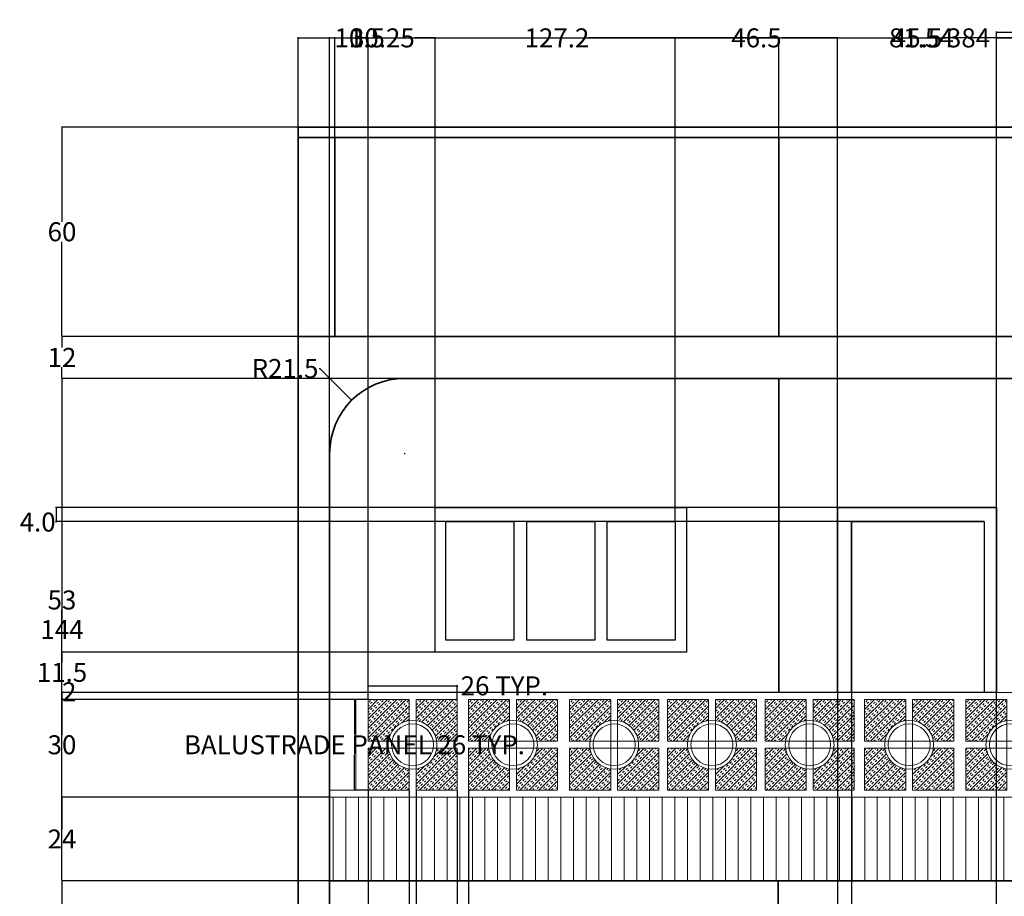
# Model space of a CAD drawing. Units: inches. Extents: x 12 to 590, y 127 to 569.
# Tile 2 of 4: x 12 to 294, y 318 to 569. Entities that reach past the tile are written whole.
import ezdxf

# ---------------------------------------------------------------- set-up
doc = ezdxf.new("R2010")
doc.units = ezdxf.units.IN
doc.header["$MEASUREMENT"] = 0
for name, color, linetype, lineweight in [('A-ANNO-DIMS', 2, 'Continuous', 18), ('A-DETL-RAIL', 6, 'Continuous', 18), ('A-DOOR', 3, 'Continuous', 25), ('A-ELEV', 7, 'Continuous', 35), ('A-GLAZ', 4, 'Continuous', 25), ('A-WALL-PATT', 8, 'Continuous', 13)]:
    doc.layers.add(name, color=color, linetype=linetype, lineweight=lineweight)
doc.styles.get("Standard").update_dxf_attribs({"font": 'arial.ttf'})
doc.dimstyles.get("Standard").update_dxf_attribs({"dimtxt": 5.4375, "dimasz": 0.18, "dimexe": 0.18, "dimexo": 0.0625, "dimgap": 0.09, "dimtad": 0, "dimtih": 1, "dimtoh": 1, "dimdec": 4, "dimzin": 0, "dimdsep": 46, "dimlunit": 4, "dimtxsty": 'Standard', "dimcen": 0.09, "dimadec": 0, "dimazin": 0, "dimtfac": 1, "dimtdec": 4, "dimtofl": 0, "dimtmove": 0, "dimatfit": 3, "dimfxl": 1, "dimtolj": 1, "dimtzin": 0, "dimarcsym": 0})

# ---------------------------------------------------------------- blocks, each defined once
blk = doc.blocks.new('BALUSTRADE-PANEL')
for p, q in [((11.75, 13), (11.75, 26)), ((13.75, 13), (13.75, 26)), ((12.75, 14), (0, 14)), ((12.75, 12), (0, 12)), ((11.75, 13), (11.75, 0)), ((12.75, 14), (25.5, 14)), ((12.75, 12), (25.5, 12)), ((13.75, 13), (13.75, 0))]:
    blk.add_line(p, q)
for points in [[(0, 14), (0, 26), (11.75, 26)], [(13.75, 26), (25.5, 26), (25.5, 14)], [(11.75, 0), (0, 0), (0, 12)], [(25.5, 12), (25.5, 0), (13.75, 0)]]:
    blk.add_lwpolyline(points)
for radius in [7, 6]:
    blk.add_circle((12.75, 13), radius)
blk = doc.blocks.new('WIN-3PANE')
for points in [[(0, 41.5), (72, 41.5), (72, 0), (0, 0)], [(3, 37.5), (22.5, 37.5), (22.5, 3.5), (3, 3.5)], [(26.25, 37.5), (45.75, 37.5), (45.75, 3.5), (26.25, 3.5)], [(49.25, 37.5), (68.75, 37.5), (68.75, 3.5), (49.25, 3.5)]]:
    blk.add_lwpolyline(points, close=True)
blk = doc.blocks.new('*D5')
at = {"layer": 'A-ANNO-DIMS', "color": 0, "lineweight": -2, "transparency": 16777216}
for p, q in [((111.44, 374), (107.42, 374)), ((107.6, 373.82), (107.6, 363.9)), ((107.6, 348.18), (107.6, 358.1)), ((111.44, 348), (107.42, 348))]:
    blk.add_line(p, q, dxfattribs=at)
at = {"layer": 'A-ANNO-DIMS', "color": 0, "transparency": 16777216}
for points in [[(107.57, 373.82), (107.63, 373.82), (107.6, 374)], [(107.57, 348.18), (107.63, 348.18), (107.6, 348)]]:
    blk.add_solid(points, dxfattribs=at)
at = {"layer": 'Defpoints', "color": 0, "transparency": 16777216}
for p in [(107.6, 374), (111.5, 374), (111.5, 348)]:
    blk.add_point(p, dxfattribs=at)
at = {"layer": 'A-ANNO-DIMS', "color": 0, "transparency": 16777216, "insert": (107.6, 361), "char_height": 5.4375, "attachment_point": 5}
blk.add_mtext('\\A1;BALUSTRADE PANEL 26 TYP.', dxfattribs=at)
blk = doc.blocks.new('*D6')
at = {"layer": 'A-ANNO-DIMS', "color": 0, "lineweight": -2, "transparency": 16777216}
for p, q in [((111.5, 374.06), (111.5, 378.08)), ((137, 374.06), (137, 378.08)), ((111.68, 377.9), (136.82, 377.9)), ((137, 377.9), (137.18, 377.9))]:
    blk.add_line(p, q, dxfattribs=at)
at = {"layer": 'A-ANNO-DIMS', "color": 0, "transparency": 16777216}
for points in [[(111.68, 377.93), (111.68, 377.87), (111.5, 377.9)], [(136.82, 377.93), (136.82, 377.87), (137, 377.9)]]:
    blk.add_solid(points, dxfattribs=at)
at = {"layer": 'Defpoints', "color": 0, "transparency": 16777216}
for p in [(137, 377.9), (111.5, 374), (137, 374)]:
    blk.add_point(p, dxfattribs=at)
at = {"layer": 'A-ANNO-DIMS', "color": 0, "transparency": 16777216, "insert": (150.55, 377.9), "char_height": 5.4375, "attachment_point": 5}
blk.add_mtext('\\A1;26 TYP.', dxfattribs=at)
blk = doc.blocks.new('*D7')
at = {"layer": 'A-ANNO-DIMS', "color": 0, "lineweight": -2, "transparency": 16777216}
for p, q in [((91.5, 538.06), (91.5, 563.73)), ((91.68, 563.55), (277.42, 563.55)), ((475.32, 563.55), (289.58, 563.55)), ((475.5, 538.06), (475.5, 563.73))]:
    blk.add_line(p, q, dxfattribs=at)
at = {"layer": 'A-ANNO-DIMS', "color": 0, "transparency": 16777216}
for points in [[(91.68, 563.58), (91.68, 563.52), (91.5, 563.55)], [(475.32, 563.58), (475.32, 563.52), (475.5, 563.55)]]:
    blk.add_solid(points, dxfattribs=at)
at = {"layer": 'Defpoints', "color": 0, "transparency": 16777216}
for p in [(475.5, 563.55), (91.5, 538), (475.5, 538)]:
    blk.add_point(p, dxfattribs=at)
at = {"layer": 'A-ANNO-DIMS', "color": 0, "transparency": 16777216, "insert": (283.5, 563.55), "char_height": 5.438, "attachment_point": 5}
blk.add_mtext('\\A1;384', dxfattribs=at)
blk = doc.blocks.new('*D9')
at = {"layer": 'A-ANNO-DIMS', "color": 0, "lineweight": -2, "transparency": 16777216}
for p, q in [((91.5, 535.06), (91.5, 563.73)), ((91.68, 563.55), (101.82, 563.55)), ((102, 535.06), (102, 563.73)), ((102, 563.55), (102.18, 563.55))]:
    blk.add_line(p, q, dxfattribs=at)
at = {"layer": 'A-ANNO-DIMS', "color": 0, "transparency": 16777216}
for points in [[(91.68, 563.58), (91.68, 563.52), (91.5, 563.55)], [(101.82, 563.58), (101.82, 563.52), (102, 563.55)]]:
    blk.add_solid(points, dxfattribs=at)
at = {"layer": 'Defpoints', "color": 0, "transparency": 16777216}
for p in [(102, 563.55), (91.5, 535), (102, 535)]:
    blk.add_point(p, dxfattribs=at)
at = {"layer": 'A-ANNO-DIMS', "color": 0, "transparency": 16777216, "insert": (109.1, 563.55), "char_height": 5.438, "attachment_point": 5}
blk.add_mtext('\\A1;10.5', dxfattribs=at)
blk = doc.blocks.new('*D10')
at = {"layer": 'A-ANNO-DIMS', "color": 0, "lineweight": -2, "transparency": 16777216}
for p, q in [((102, 535.06), (102, 563.73)), ((102.18, 563.55), (156.62, 563.55)), ((229.03, 563.55), (174.59, 563.55)), ((229.21, 535.06), (229.21, 563.73))]:
    blk.add_line(p, q, dxfattribs=at)
at = {"layer": 'A-ANNO-DIMS', "color": 0, "transparency": 16777216}
for points in [[(102.18, 563.58), (102.18, 563.52), (102, 563.55)], [(229.03, 563.58), (229.03, 563.52), (229.21, 563.55)]]:
    blk.add_solid(points, dxfattribs=at)
at = {"layer": 'Defpoints', "color": 0, "transparency": 16777216}
for p in [(229.21, 563.55), (102, 535), (229.21, 535)]:
    blk.add_point(p, dxfattribs=at)
at = {"layer": 'A-ANNO-DIMS', "color": 0, "transparency": 16777216, "insert": (165.61, 563.55), "char_height": 5.438, "attachment_point": 5}
blk.add_mtext('\\A1;127.2', dxfattribs=at)
blk = doc.blocks.new('*D11')
at = {"layer": 'A-ANNO-DIMS', "color": 0, "lineweight": -2, "transparency": 16777216}
for p, q in [((229.21, 535.06), (229.21, 563.73)), ((229.39, 563.55), (260.72, 563.55)), ((310.57, 563.55), (279.24, 563.55)), ((310.75, 535.06), (310.75, 563.73))]:
    blk.add_line(p, q, dxfattribs=at)
at = {"layer": 'A-ANNO-DIMS', "color": 0, "transparency": 16777216}
for points in [[(229.39, 563.58), (229.39, 563.52), (229.21, 563.55)], [(310.57, 563.58), (310.57, 563.52), (310.75, 563.55)]]:
    blk.add_solid(points, dxfattribs=at)
at = {"layer": 'Defpoints', "color": 0, "transparency": 16777216}
for p in [(310.75, 563.55), (229.21, 535), (310.75, 535)]:
    blk.add_point(p, dxfattribs=at)
at = {"layer": 'A-ANNO-DIMS', "color": 0, "transparency": 16777216, "insert": (269.98, 563.55), "char_height": 5.438, "attachment_point": 5}
blk.add_mtext('\\A1;81.54', dxfattribs=at)
blk = doc.blocks.new('*D17')
at = {"layer": 'A-ANNO-DIMS', "color": 0, "lineweight": -2, "transparency": 16777216}
for p, q in [((121.94, 466), (23.66, 466)), ((23.84, 465.82), (23.84, 396.82)), ((23.84, 322.18), (23.84, 391.18)), ((100.44, 322), (23.66, 322))]:
    blk.add_line(p, q, dxfattribs=at)
at = {"layer": 'A-ANNO-DIMS', "color": 0, "transparency": 16777216}
for points in [[(23.81, 465.82), (23.87, 465.82), (23.84, 466)], [(23.81, 322.18), (23.87, 322.18), (23.84, 322)]]:
    blk.add_solid(points, dxfattribs=at)
at = {"layer": 'Defpoints', "color": 0, "transparency": 16777216}
for p in [(23.84, 466), (122, 466), (100.5, 322)]:
    blk.add_point(p, dxfattribs=at)
at = {"layer": 'A-ANNO-DIMS', "color": 0, "transparency": 16777216, "insert": (23.84, 394), "char_height": 5.438, "attachment_point": 5}
blk.add_mtext('\\A1;144', dxfattribs=at)
blk = doc.blocks.new('*D18')
at = {"layer": 'A-ANNO-DIMS', "color": 0, "lineweight": -2, "transparency": 16777216}
for p, q in [((91.44, 478), (23.66, 478)), ((23.84, 477.82), (23.84, 474.82)), ((23.84, 466.18), (23.84, 469.18)), ((121.94, 466), (23.66, 466))]:
    blk.add_line(p, q, dxfattribs=at)
at = {"layer": 'A-ANNO-DIMS', "color": 0, "transparency": 16777216}
for points in [[(23.81, 477.82), (23.87, 477.82), (23.84, 478)], [(23.81, 466.18), (23.87, 466.18), (23.84, 466)]]:
    blk.add_solid(points, dxfattribs=at)
at = {"layer": 'Defpoints', "color": 0, "transparency": 16777216}
for p in [(23.84, 478), (91.5, 478), (122, 466)]:
    blk.add_point(p, dxfattribs=at)
at = {"layer": 'A-ANNO-DIMS', "color": 0, "transparency": 16777216, "insert": (23.84, 472), "char_height": 5.438, "attachment_point": 5}
blk.add_mtext('\\A1;12', dxfattribs=at)
blk = doc.blocks.new('*D19')
at = {"layer": 'A-ANNO-DIMS', "color": 0, "lineweight": -2, "transparency": 16777216}
for p, q in [((91.44, 538), (23.66, 538)), ((23.84, 537.82), (23.84, 510.87)), ((23.84, 478.18), (23.84, 505.13)), ((91.44, 478), (23.66, 478))]:
    blk.add_line(p, q, dxfattribs=at)
at = {"layer": 'A-ANNO-DIMS', "color": 0, "transparency": 16777216}
for points in [[(23.81, 537.82), (23.87, 537.82), (23.84, 538)], [(23.81, 478.18), (23.87, 478.18), (23.84, 478)]]:
    blk.add_solid(points, dxfattribs=at)
at = {"layer": 'Defpoints', "color": 0, "transparency": 16777216}
for p in [(23.84, 538), (91.5, 538), (91.5, 478)]:
    blk.add_point(p, dxfattribs=at)
at = {"layer": 'A-ANNO-DIMS', "color": 0, "transparency": 16777216, "insert": (23.84, 508), "char_height": 5.438, "attachment_point": 5}
blk.add_mtext('\\A1;60', dxfattribs=at)
blk = doc.blocks.new('*D28')
at = {"layer": 'A-ANNO-DIMS', "color": 0, "lineweight": -2, "transparency": 16777216}
for p, q in [((291.5, 429.06), (291.5, 563.73)), ((291.68, 563.55), (317.01, 563.55)), ((350.32, 563.55), (324.99, 563.55)), ((350.5, 429.06), (350.5, 563.73))]:
    blk.add_line(p, q, dxfattribs=at)
at = {"layer": 'A-ANNO-DIMS', "color": 0, "transparency": 16777216}
for points in [[(291.68, 563.58), (291.68, 563.52), (291.5, 563.55)], [(350.32, 563.58), (350.32, 563.52), (350.5, 563.55)]]:
    blk.add_solid(points, dxfattribs=at)
at = {"layer": 'Defpoints', "color": 0, "transparency": 16777216}
for p in [(350.5, 563.55), (291.5, 429), (350.5, 429)]:
    blk.add_point(p, dxfattribs=at)
at = {"layer": 'A-ANNO-DIMS', "color": 0, "transparency": 16777216, "insert": (321, 563.55), "char_height": 5.438, "attachment_point": 5}
blk.add_mtext('\\A1;59', dxfattribs=at)
blk = doc.blocks.new('*D30')
at = {"layer": 'A-ANNO-DIMS', "color": 0, "lineweight": -2, "transparency": 16777216}
for p, q in [((100.44, 322), (23.66, 322)), ((23.84, 321.82), (23.84, 306.37)), ((23.84, 285.18), (23.84, 300.63)), ((130.69, 285), (23.66, 285))]:
    blk.add_line(p, q, dxfattribs=at)
at = {"layer": 'A-ANNO-DIMS', "color": 0, "transparency": 16777216}
for points in [[(23.81, 321.82), (23.87, 321.82), (23.84, 322)], [(23.81, 285.18), (23.87, 285.18), (23.84, 285)]]:
    blk.add_solid(points, dxfattribs=at)
at = {"layer": 'Defpoints', "color": 0, "transparency": 16777216}
for p in [(23.84, 322), (100.5, 322), (130.75, 285)]:
    blk.add_point(p, dxfattribs=at)
at = {"layer": 'A-ANNO-DIMS', "color": 0, "transparency": 16777216, "insert": (23.84, 303.5), "char_height": 5.438, "attachment_point": 5}
blk.add_mtext('\\A1;37', dxfattribs=at)
blk = doc.blocks.new('*D32')
at = {"layer": 'A-ANNO-DIMS', "color": 0, "lineweight": -2, "transparency": 16777216}
for p, q in [((100.5, 444.56), (100.5, 563.73)), ((100.68, 563.55), (106.34, 563.55)), ((130.57, 563.55), (124.91, 563.55)), ((130.75, 429.06), (130.75, 563.73))]:
    blk.add_line(p, q, dxfattribs=at)
at = {"layer": 'A-ANNO-DIMS', "color": 0, "transparency": 16777216}
for points in [[(100.68, 563.58), (100.68, 563.52), (100.5, 563.55)], [(130.57, 563.58), (130.57, 563.52), (130.75, 563.55)]]:
    blk.add_solid(points, dxfattribs=at)
at = {"layer": 'Defpoints', "color": 0, "transparency": 16777216}
for p in [(130.75, 563.55), (100.5, 444.5), (130.75, 429)]:
    blk.add_point(p, dxfattribs=at)
at = {"layer": 'A-ANNO-DIMS', "color": 0, "transparency": 16777216, "insert": (115.62, 563.55), "char_height": 5.438, "attachment_point": 5}
blk.add_mtext('\\A1;30.25', dxfattribs=at)
blk = doc.blocks.new('*D33')
at = {"layer": 'A-ANNO-DIMS', "color": 0, "lineweight": -2, "transparency": 16777216}
for p, q in [((199.5, 425.06), (199.5, 563.73)), ((199.68, 563.55), (215.47, 563.55)), ((245.82, 563.55), (230.03, 563.55)), ((246, 429.06), (246, 563.73))]:
    blk.add_line(p, q, dxfattribs=at)
at = {"layer": 'A-ANNO-DIMS', "color": 0, "transparency": 16777216}
for points in [[(199.68, 563.58), (199.68, 563.52), (199.5, 563.55)], [(245.82, 563.58), (245.82, 563.52), (246, 563.55)]]:
    blk.add_solid(points, dxfattribs=at)
at = {"layer": 'Defpoints', "color": 0, "transparency": 16777216}
for p in [(246, 563.55), (246, 429), (199.5, 425)]:
    blk.add_point(p, dxfattribs=at)
at = {"layer": 'A-ANNO-DIMS', "color": 0, "transparency": 16777216, "insert": (222.75, 563.55), "char_height": 5.438, "attachment_point": 5}
blk.add_mtext('\\A1;46.5', dxfattribs=at)
blk = doc.blocks.new('*D34')
at = {"layer": 'A-ANNO-DIMS', "color": 0, "lineweight": -2, "transparency": 16777216}
for p, q in [((246, 429.06), (246, 563.73)), ((246.18, 563.55), (261.47, 563.55)), ((291.32, 563.55), (276.03, 563.55)), ((291.5, 429.06), (291.5, 563.73))]:
    blk.add_line(p, q, dxfattribs=at)
at = {"layer": 'A-ANNO-DIMS', "color": 0, "transparency": 16777216}
for points in [[(246.18, 563.58), (246.18, 563.52), (246, 563.55)], [(291.32, 563.58), (291.32, 563.52), (291.5, 563.55)]]:
    blk.add_solid(points, dxfattribs=at)
at = {"layer": 'Defpoints', "color": 0, "transparency": 16777216}
for p in [(291.5, 563.55), (246, 429), (291.5, 429)]:
    blk.add_point(p, dxfattribs=at)
at = {"layer": 'A-ANNO-DIMS', "color": 0, "transparency": 16777216, "insert": (268.75, 563.55), "char_height": 5.438, "attachment_point": 5}
blk.add_mtext('\\A1;45.5', dxfattribs=at)
blk = doc.blocks.new('*D35')
at = {"layer": 'A-ANNO-DIMS', "color": 0, "lineweight": -2, "transparency": 16777216}
for p, q in [((130.69, 387.5), (23.66, 387.5)), ((23.84, 387.32), (23.84, 384.62)), ((23.84, 376.18), (23.84, 378.88)), ((100.44, 376), (23.66, 376))]:
    blk.add_line(p, q, dxfattribs=at)
at = {"layer": 'A-ANNO-DIMS', "color": 0, "transparency": 16777216}
for points in [[(23.81, 387.32), (23.87, 387.32), (23.84, 387.5)], [(23.81, 376.18), (23.87, 376.18), (23.84, 376)]]:
    blk.add_solid(points, dxfattribs=at)
at = {"layer": 'Defpoints', "color": 0, "transparency": 16777216}
for p in [(23.84, 387.5), (130.75, 387.5), (100.5, 376)]:
    blk.add_point(p, dxfattribs=at)
at = {"layer": 'A-ANNO-DIMS', "color": 0, "transparency": 16777216, "insert": (23.84, 381.75), "char_height": 5.438, "attachment_point": 5}
blk.add_mtext('\\A1;11.5', dxfattribs=at)
blk = doc.blocks.new('*D36')
at = {"layer": 'A-ANNO-DIMS', "color": 0, "lineweight": -2, "transparency": 16777216}
for p, q in [((245.94, 429), (23.66, 429)), ((23.84, 428.82), (23.84, 405.37)), ((23.84, 376.18), (23.84, 399.63)), ((249.94, 376), (23.66, 376))]:
    blk.add_line(p, q, dxfattribs=at)
at = {"layer": 'A-ANNO-DIMS', "color": 0, "transparency": 16777216}
for points in [[(23.81, 428.82), (23.87, 428.82), (23.84, 429)], [(23.81, 376.18), (23.87, 376.18), (23.84, 376)]]:
    blk.add_solid(points, dxfattribs=at)
at = {"layer": 'Defpoints', "color": 0, "transparency": 16777216}
for p in [(23.84, 429), (246, 429), (250, 376)]:
    blk.add_point(p, dxfattribs=at)
at = {"layer": 'A-ANNO-DIMS', "color": 0, "transparency": 16777216, "insert": (23.84, 402.5), "char_height": 5.438, "attachment_point": 5}
blk.add_mtext('\\A1;53', dxfattribs=at)
blk = doc.blocks.new('*D37')
at = {"layer": 'A-ANNO-DIMS', "color": 0, "lineweight": -2, "transparency": 16777216}
for p, q in [((100.44, 346), (23.66, 346)), ((23.84, 345.82), (23.84, 336.82)), ((23.84, 322.18), (23.84, 331.18)), ((100.44, 322), (23.66, 322))]:
    blk.add_line(p, q, dxfattribs=at)
at = {"layer": 'A-ANNO-DIMS', "color": 0, "transparency": 16777216}
for points in [[(23.81, 345.82), (23.87, 345.82), (23.84, 346)], [(23.81, 322.18), (23.87, 322.18), (23.84, 322)]]:
    blk.add_solid(points, dxfattribs=at)
at = {"layer": 'Defpoints', "color": 0, "transparency": 16777216}
for p in [(23.84, 346), (100.5, 346), (100.5, 322)]:
    blk.add_point(p, dxfattribs=at)
at = {"layer": 'A-ANNO-DIMS', "color": 0, "transparency": 16777216, "insert": (23.84, 334), "char_height": 5.438, "attachment_point": 5}
blk.add_mtext('\\A1;24', dxfattribs=at)
blk = doc.blocks.new('*D38')
at = {"layer": 'A-ANNO-DIMS', "color": 0, "lineweight": -2, "transparency": 16777216}
for p, q in [((100.44, 376), (23.66, 376)), ((23.84, 375.82), (23.84, 363.87)), ((23.84, 346.18), (23.84, 358.13)), ((100.44, 346), (23.66, 346))]:
    blk.add_line(p, q, dxfattribs=at)
at = {"layer": 'A-ANNO-DIMS', "color": 0, "transparency": 16777216}
for points in [[(23.81, 375.82), (23.87, 375.82), (23.84, 376)], [(23.81, 346.18), (23.87, 346.18), (23.84, 346)]]:
    blk.add_solid(points, dxfattribs=at)
at = {"layer": 'Defpoints', "color": 0, "transparency": 16777216}
for p in [(23.84, 376), (100.5, 376), (100.5, 346)]:
    blk.add_point(p, dxfattribs=at)
at = {"layer": 'A-ANNO-DIMS', "color": 0, "transparency": 16777216, "insert": (23.84, 361), "char_height": 5.438, "attachment_point": 5}
blk.add_mtext('\\A1;30', dxfattribs=at)
blk = doc.blocks.new('*D43')
at = {"layer": 'A-ANNO-DIMS', "color": 0, "lineweight": -2, "transparency": 16777216}
for p, q in [((100.5, 376.06), (100.5, 563.73)), ((100.68, 563.55), (102.8, 563.55)), ((111.32, 563.55), (109.2, 563.55)), ((111.5, 374.06), (111.5, 563.73))]:
    blk.add_line(p, q, dxfattribs=at)
at = {"layer": 'A-ANNO-DIMS', "color": 0, "transparency": 16777216}
for points in [[(100.68, 563.58), (100.68, 563.52), (100.5, 563.55)], [(111.32, 563.58), (111.32, 563.52), (111.5, 563.55)]]:
    blk.add_solid(points, dxfattribs=at)
at = {"layer": 'Defpoints', "color": 0, "transparency": 16777216}
for p in [(111.5, 563.55), (100.5, 376), (111.5, 374)]:
    blk.add_point(p, dxfattribs=at)
at = {"layer": 'A-ANNO-DIMS', "color": 0, "transparency": 16777216, "insert": (106, 563.55), "char_height": 5.438, "attachment_point": 5}
blk.add_mtext('\\A1;11', dxfattribs=at)
blk = doc.blocks.new('*D44')
at = {"layer": 'A-ANNO-DIMS', "color": 0, "lineweight": -2, "transparency": 16777216}
for p, q in [((111.5, 347.94), (111.5, 131.59)), ((123.25, 347.94), (123.25, 131.59)), ((111.68, 131.77), (123.07, 131.77)), ((123.25, 131.77), (123.43, 131.77))]:
    blk.add_line(p, q, dxfattribs=at)
at = {"layer": 'A-ANNO-DIMS', "color": 0, "transparency": 16777216}
for points in [[(111.68, 131.8), (111.68, 131.74), (111.5, 131.77)], [(123.07, 131.8), (123.07, 131.74), (123.25, 131.77)]]:
    blk.add_solid(points, dxfattribs=at)
at = {"layer": 'Defpoints', "color": 0, "transparency": 16777216}
for p in [(111.5, 348), (123.25, 348), (123.25, 131.77)]:
    blk.add_point(p, dxfattribs=at)
at = {"layer": 'A-ANNO-DIMS', "color": 0, "transparency": 16777216, "insert": (132.46, 131.77), "char_height": 5.438, "attachment_point": 5}
blk.add_mtext('\\A1;11.75', dxfattribs=at)
blk = doc.blocks.new('*D45')
at = {"layer": 'A-ANNO-DIMS', "color": 0, "lineweight": -2, "transparency": 16777216}
for p, q in [((123.25, 347.94), (123.25, 131.59)), ((125.25, 347.94), (125.25, 131.59)), ((123.43, 131.77), (125.07, 131.77)), ((125.25, 131.77), (125.43, 131.77))]:
    blk.add_line(p, q, dxfattribs=at)
at = {"layer": 'A-ANNO-DIMS', "color": 0, "transparency": 16777216}
for points in [[(123.43, 131.8), (123.43, 131.74), (123.25, 131.77)], [(125.07, 131.8), (125.07, 131.74), (125.25, 131.77)]]:
    blk.add_solid(points, dxfattribs=at)
at = {"layer": 'Defpoints', "color": 0, "transparency": 16777216}
for p in [(123.25, 348), (125.25, 348), (125.25, 131.77)]:
    blk.add_point(p, dxfattribs=at)
at = {"layer": 'A-ANNO-DIMS', "color": 0, "transparency": 16777216, "insert": (127.32, 131.77), "char_height": 5.438, "attachment_point": 5}
blk.add_mtext('\\A1;2', dxfattribs=at)
blk = doc.blocks.new('*D46')
at = {"layer": 'A-ANNO-DIMS', "color": 0, "lineweight": -2, "transparency": 16777216}
for p, q in [((137, 347.94), (137, 131.59)), ((140.25, 347.94), (140.25, 131.59)), ((137.18, 131.77), (140.07, 131.77)), ((140.25, 131.77), (140.43, 131.77))]:
    blk.add_line(p, q, dxfattribs=at)
at = {"layer": 'A-ANNO-DIMS', "color": 0, "transparency": 16777216}
for points in [[(137.18, 131.8), (137.18, 131.74), (137, 131.77)], [(140.07, 131.8), (140.07, 131.74), (140.25, 131.77)]]:
    blk.add_solid(points, dxfattribs=at)
at = {"layer": 'Defpoints', "color": 0, "transparency": 16777216}
for p in [(137, 348), (140.25, 348), (140.25, 131.77)]:
    blk.add_point(p, dxfattribs=at)
at = {"layer": 'A-ANNO-DIMS', "color": 0, "transparency": 16777216, "insert": (147.6, 131.77), "char_height": 5.438, "attachment_point": 5}
blk.add_mtext('\\A1;3.25', dxfattribs=at)
blk = doc.blocks.new('*D47')
at = {"layer": 'A-ANNO-DIMS', "color": 0, "lineweight": -2, "transparency": 16777216}
for p, q in [((100.44, 376), (23.66, 376)), ((23.84, 376), (23.84, 376.18)), ((23.84, 376.18), (24.02, 376.18)), ((23.84, 374.18), (23.84, 375.82)), ((111.44, 374), (23.66, 374))]:
    blk.add_line(p, q, dxfattribs=at)
at = {"layer": 'A-ANNO-DIMS', "color": 0, "transparency": 16777216}
for points in [[(23.81, 375.82), (23.87, 375.82), (23.84, 376)], [(23.81, 374.18), (23.87, 374.18), (23.84, 374)]]:
    blk.add_solid(points, dxfattribs=at)
at = {"layer": 'Defpoints', "color": 0, "transparency": 16777216}
for p in [(23.84, 376), (100.5, 376), (111.5, 374)]:
    blk.add_point(p, dxfattribs=at)
at = {"layer": 'A-ANNO-DIMS', "color": 0, "transparency": 16777216, "insert": (25.91, 376.18), "char_height": 5.438, "attachment_point": 5}
blk.add_mtext('\\A1;2', dxfattribs=at)
blk = doc.blocks.new('*D53')
at = {"layer": 'A-ANNO-DIMS', "color": 0, "lineweight": -2, "transparency": 16777216}
for p, q in [((97.5, 468.82), (97.68, 468.82)), ((97.68, 468.82), (106.67, 459.83)), ((121.91, 444.5), (122.09, 444.5)), ((122, 444.41), (122, 444.59))]:
    blk.add_line(p, q, dxfattribs=at)
at = {"layer": 'A-ANNO-DIMS', "color": 0, "transparency": 16777216}
blk.add_solid([(106.69, 459.85), (106.65, 459.81), (106.8, 459.7)], dxfattribs=at)
at = {"layer": 'Defpoints', "color": 0, "transparency": 16777216}
for p in [(106.8, 459.7), (122, 444.5)]:
    blk.add_point(p, dxfattribs=at)
at = {"layer": 'A-ANNO-DIMS', "color": 0, "transparency": 16777216, "insert": (87.72, 468.82), "char_height": 5.438, "attachment_point": 5}
blk.add_mtext('\\A1;R21.5', dxfattribs=at)
blk = doc.blocks.new('*D58')
at = {"layer": 'A-ANNO-DIMS', "color": 0, "lineweight": -2, "transparency": 16777216}
for p, q in [((246, 428.94), (246, 129.94)), ((250, 424.94), (250, 129.94)), ((246.18, 130.12), (249.82, 130.12)), ((250, 130.12), (250.18, 130.12))]:
    blk.add_line(p, q, dxfattribs=at)
at = {"layer": 'A-ANNO-DIMS', "color": 0, "transparency": 16777216}
for points in [[(246.18, 130.15), (246.18, 130.09), (246, 130.12)], [(249.82, 130.15), (249.82, 130.09), (250, 130.12)]]:
    blk.add_solid(points, dxfattribs=at)
at = {"layer": 'Defpoints', "color": 0, "transparency": 16777216}
for p in [(246, 429), (250, 425), (250, 130.12)]:
    blk.add_point(p, dxfattribs=at)
at = {"layer": 'A-ANNO-DIMS', "color": 0, "transparency": 16777216, "insert": (255.32, 130.12), "char_height": 5.438, "attachment_point": 5}
blk.add_mtext('\\A1;4.0', dxfattribs=at)
blk = doc.blocks.new('*D59')
at = {"layer": 'A-ANNO-DIMS', "color": 0, "lineweight": -2, "transparency": 16777216}
for p, q in [((291.44, 429), (22.01, 429)), ((22.19, 428.82), (22.19, 425.18)), ((287.94, 425), (22.01, 425)), ((22.19, 424.82), (22.01, 424.82)), ((22.19, 425), (22.19, 424.82))]:
    blk.add_line(p, q, dxfattribs=at)
at = {"layer": 'A-ANNO-DIMS', "color": 0, "transparency": 16777216}
for points in [[(22.16, 428.82), (22.22, 428.82), (22.19, 429)], [(22.16, 425.18), (22.22, 425.18), (22.19, 425)]]:
    blk.add_solid(points, dxfattribs=at)
at = {"layer": 'Defpoints', "color": 0, "transparency": 16777216}
for p in [(291.5, 429), (22.19, 425), (288, 425)]:
    blk.add_point(p, dxfattribs=at)
at = {"layer": 'A-ANNO-DIMS', "color": 0, "transparency": 16777216, "insert": (16.87, 424.82), "char_height": 5.438, "attachment_point": 5}
blk.add_mtext('\\A1;4.0', dxfattribs=at)
blk = doc.blocks.new('*D60')
at = {"layer": 'A-ANNO-DIMS', "color": 0, "lineweight": -2, "transparency": 16777216}
for p, q in [((291.5, 285.06), (291.5, 565.38)), ((291.68, 565.2), (313.86, 565.2)), ((350.32, 565.2), (328.14, 565.2)), ((350.5, 285.06), (350.5, 565.38))]:
    blk.add_line(p, q, dxfattribs=at)
at = {"layer": 'A-ANNO-DIMS', "color": 0, "transparency": 16777216}
for points in [[(291.68, 565.23), (291.68, 565.17), (291.5, 565.2)], [(350.32, 565.23), (350.32, 565.17), (350.5, 565.2)]]:
    blk.add_solid(points, dxfattribs=at)
at = {"layer": 'Defpoints', "color": 0, "transparency": 16777216}
for p in [(350.5, 565.2), (291.5, 285), (350.5, 285)]:
    blk.add_point(p, dxfattribs=at)
at = {"layer": 'A-ANNO-DIMS', "color": 0, "transparency": 16777216, "insert": (321, 565.2), "char_height": 5.438, "attachment_point": 5}
blk.add_mtext('\\A1;59.0', dxfattribs=at)

msp = doc.modelspace()

# ---------------------------------------------------------------- hatches: boundary and pattern name
at = {"layer": 'A-WALL-PATT'}
h = msp.add_hatch(dxfattribs=at)
h.set_pattern_fill('INSUL', color=256, scale=5.1, angle=45)
h.paths.add_polyline_path([(123.25, 374), (111.5, 374), (111.5, 362), (117.3218, 362, -0.33252769), (123.25, 367.9282)])
h.paths.add_polyline_path([(137, 374), (125.25, 374), (125.25, 367.9282, -0.33252769), (131.1782, 362), (137, 362)])
h.paths.add_polyline_path([(137, 360), (131.1782, 360, -0.33252769), (125.25, 354.0718), (125.25, 348), (137, 348)])
h.paths.add_polyline_path([(123.25, 354.0718, -0.33252769), (117.3218, 360), (111.5, 360), (111.5, 348), (123.25, 348)])
h = msp.add_hatch(dxfattribs=at)
h.set_pattern_fill('INSUL', color=256, scale=5.1, angle=45)
h.set_pattern_definition([(45, (28.75, 0), (-1.352342, 1.352342), []), (45, (28.2992, 0.4508), (-1.352342, 1.352342), [0.6375, -0.6375]), (45, (27.8484, 0.9016), (-1.352342, 1.352342), [0.6375, -0.6375])])
h.paths.add_polyline_path([(152, 374), (140.25, 374), (140.25, 362), (146.0718, 362, -0.33252769), (152, 367.9282)])
h.paths.add_polyline_path([(165.75, 374), (154, 374), (154, 367.9282, -0.33252769), (159.9282, 362), (165.75, 362)])
h.paths.add_polyline_path([(165.75, 360), (159.9282, 360, -0.33252769), (154, 354.0718), (154, 348), (165.75, 348)])
h.paths.add_polyline_path([(152, 354.0718, -0.33252769), (146.0718, 360), (140.25, 360), (140.25, 348), (152, 348)])
h = msp.add_hatch(dxfattribs=at)
h.set_pattern_fill('INSUL', color=256, scale=5.1, angle=45)
h.set_pattern_definition([(45, (57.75, 0), (-1.352342, 1.352342), []), (45, (57.2992, 0.4508), (-1.352342, 1.352342), [0.6375, -0.6375]), (45, (56.8484, 0.9016), (-1.352342, 1.352342), [0.6375, -0.6375])])
h.paths.add_polyline_path([(181, 374), (169.25, 374), (169.25, 362), (175.0718, 362, -0.33252769), (181, 367.9282)])
h.paths.add_polyline_path([(194.75, 374), (183, 374), (183, 367.9282, -0.33252769), (188.9282, 362), (194.75, 362)])
h.paths.add_polyline_path([(194.75, 360), (188.9282, 360, -0.33252769), (183, 354.0718), (183, 348), (194.75, 348)])
h.paths.add_polyline_path([(181, 354.0718, -0.33252769), (175.0718, 360), (169.25, 360), (169.25, 348), (181, 348)])
h = msp.add_hatch(dxfattribs=at)
h.set_pattern_fill('INSUL', color=256, scale=5.1, angle=45)
h.set_pattern_definition([(45, (85.75, 0), (-1.352342, 1.352342), []), (45, (85.2992, 0.4508), (-1.352342, 1.352342), [0.6375, -0.6375]), (45, (84.8484, 0.9016), (-1.352342, 1.352342), [0.6375, -0.6375])])
h.paths.add_polyline_path([(209, 374), (197.25, 374), (197.25, 362), (203.0718, 362, -0.33252769), (209, 367.9282)])
h.paths.add_polyline_path([(222.75, 374), (211, 374), (211, 367.9282, -0.33252769), (216.9282, 362), (222.75, 362)])
h.paths.add_polyline_path([(222.75, 360), (216.9282, 360, -0.33252769), (211, 354.0718), (211, 348), (222.75, 348)])
h.paths.add_polyline_path([(209, 354.0718, -0.33252769), (203.0718, 360), (197.25, 360), (197.25, 348), (209, 348)])
h = msp.add_hatch(dxfattribs=at)
h.set_pattern_fill('INSUL', color=256, scale=5.1, angle=45)
h.set_pattern_definition([(45, (113.75, 0), (-1.352342, 1.352342), []), (45, (113.2992, 0.4508), (-1.352342, 1.352342), [0.6375, -0.6375]), (45, (112.8484, 0.9016), (-1.352342, 1.352342), [0.6375, -0.6375])])
h.paths.add_polyline_path([(237, 374), (225.25, 374), (225.25, 362), (231.0718, 362, -0.33252769), (237, 367.9282)])
h.paths.add_polyline_path([(250.75, 374), (239, 374), (239, 367.9282, -0.33252769), (244.9282, 362), (250.75, 362)])
h.paths.add_polyline_path([(250.75, 360), (244.9282, 360, -0.33252769), (239, 354.0718), (239, 348), (250.75, 348)])
h.paths.add_polyline_path([(237, 354.0718, -0.33252769), (231.0718, 360), (225.25, 360), (225.25, 348), (237, 348)])
h = msp.add_hatch(dxfattribs=at)
h.set_pattern_fill('INSUL', color=256, scale=5.1, angle=45)
h.set_pattern_definition([(45, (142.25, 0), (-1.352342, 1.352342), []), (45, (141.7992, 0.4508), (-1.352342, 1.352342), [0.6375, -0.6375]), (45, (141.3484, 0.9016), (-1.352342, 1.352342), [0.6375, -0.6375])])
h.paths.add_polyline_path([(265.5, 374), (253.75, 374), (253.75, 362), (259.5718, 362, -0.33252769), (265.5, 367.9282)])
h.paths.add_polyline_path([(279.25, 374), (267.5, 374), (267.5, 367.9282, -0.33252769), (273.4282, 362), (279.25, 362)])
h.paths.add_polyline_path([(279.25, 360), (273.4282, 360, -0.33252769), (267.5, 354.0718), (267.5, 348), (279.25, 348)])
h.paths.add_polyline_path([(265.5, 354.0718, -0.33252769), (259.5718, 360), (253.75, 360), (253.75, 348), (265.5, 348)])
h = msp.add_hatch(dxfattribs=at)
h.set_pattern_fill('INSUL', color=256, scale=5.1, angle=45)
h.set_pattern_definition([(45, (171.25, 0), (-1.352342, 1.352342), []), (45, (170.7992, 0.4508), (-1.352342, 1.352342), [0.6375, -0.6375]), (45, (170.3484, 0.9016), (-1.352342, 1.352342), [0.6375, -0.6375])])
h.paths.add_polyline_path([(294.5, 374), (282.75, 374), (282.75, 362), (288.5718, 362, -0.33252769), (294.5, 367.9282)])
h.paths.add_polyline_path([(308.25, 374), (296.5, 374), (296.5, 367.9282, -0.33252769), (302.4282, 362), (308.25, 362)])
h.paths.add_polyline_path([(308.25, 360), (302.4282, 360, -0.33252769), (296.5, 354.0718), (296.5, 348), (308.25, 348)])
h.paths.add_polyline_path([(294.5, 354.0718, -0.33252769), (288.5718, 360), (282.75, 360), (282.75, 348), (294.5, 348)])
h = msp.add_hatch(dxfattribs=at)
h.set_pattern_fill('ANSI31', color=256, scale=29, angle=45)
h.paths.add_polyline_path([(414, 322), (466.5, 322), (466.5, 346), (100.5, 346), (100.5, 322)])

# ---------------------------------------------------------------- linework, layer by layer
at = {"layer": 'A-DETL-RAIL'}
for p, q in [((100.5, 376), (466.5, 376)), ((100.5, 346), (466.5, 346))]:
    msp.add_line(p, q, dxfattribs=at)
msp.add_lwpolyline([(100.5, 374), (108, 374), (108, 348), (100.5, 348)], close=True, dxfattribs=at)
at = {"layer": 'A-DOOR'}
for points in [[(246, 429), (291.5, 429), (291.5, 376), (246, 376)], [(250, 425), (288, 425), (288, 376), (250, 376)]]:
    msp.add_lwpolyline(points, close=True, dxfattribs=at)
at = {"layer": 'A-ELEV'}
for p, q in [((475.5, 538), (91.5, 538)), ((91.5, 535.5), (91.5, 538)), ((91.5, 492), (91.5, 535.5)), ((102, 535), (91.5, 535)), ((102, 520), (102, 535)), ((102, 535), (466.5, 535)), ((229.2101, 478), (229.2101, 535)), ((102, 478), (102, 520)), ((91.5, 301.3163), (91.5, 492)), ((146, 478), (91.5, 478)), ((146, 478), (475.5, 478)), ((122, 466), (451.5, 466)), ((229.2101, 376), (229.2101, 466)), ((100.5, 322), (100.5, 444.5)), ((100.5, 322), (414, 322)), ((100.5, 301.3163), (100.5, 322)), ((229, 322), (228.5, 193.5))]:
    msp.add_line(p, q, dxfattribs=at)
msp.add_arc((122, 444.5), 21.5, 90, 180, dxfattribs=at)

# ---------------------------------------------------------------- block references
at = {"layer": 'A-DETL-RAIL'}
for p in [(111.5, 348), (169.25, 348), (197.25, 348), (225.25, 348), (253.75, 348), (282.75, 348)]:
    msp.add_blockref('BALUSTRADE-PANEL', p, dxfattribs=at)
at = {"layer": 'A-DETL-RAIL', "rotation": 180}
msp.add_blockref('BALUSTRADE-PANEL', (165.75, 374), dxfattribs=at)
at = {"layer": 'A-GLAZ'}
msp.add_blockref('WIN-3PANE', (130.75, 387.5), dxfattribs=at)

# ---------------------------------------------------------------- dimensions: what is measured, and where the dimension line sits
at = {"layer": 'A-ANNO-DIMS'}
for base, p1, p2, override, picture, middle in [((475.5, 563.55), (91.5, 538), (475.5, 538), {"dimdec": 0, "dimlfac": 1, "dimrnd": 0, "dimzin": 0, "dimdsep": 46, "dimlunit": 2}, '*D7', (283.5, 563.55)), ((102, 563.55), (91.5, 535), (102, 535), {"dimdec": 1, "dimlfac": 1, "dimrnd": 0, "dimzin": 0, "dimdsep": 46, "dimlunit": 2}, '*D9', (109.0965, 563.55)), ((130.75, 563.55), (100.5, 444.5), (130.75, 429), {"dimdec": 2, "dimlfac": 1, "dimrnd": 0, "dimzin": 0, "dimdsep": 46, "dimlunit": 2}, '*D32', (115.625, 563.55)), ((111.5, 563.55), (100.5, 376), (111.5, 374), {"dimdec": 0, "dimlfac": 1, "dimrnd": 0, "dimzin": 0, "dimdsep": 46, "dimlunit": 2}, '*D43', (106, 563.55)), ((229.2101, 563.55), (102, 535), (229.2101, 535), {"dimdec": 1, "dimlfac": 1, "dimrnd": 0, "dimzin": 0, "dimdsep": 46, "dimlunit": 2}, '*D10', (165.6051, 563.55)), ((246, 563.55), (199.5, 425), (246, 429), {"dimdec": 1, "dimlfac": 1, "dimrnd": 0, "dimzin": 0, "dimdsep": 46, "dimlunit": 2}, '*D33', (222.75, 563.55)), ((310.75, 563.55), (229.2101, 535), (310.75, 535), {"dimdec": 2, "dimlfac": 1, "dimrnd": 0, "dimzin": 0, "dimdsep": 46, "dimlunit": 2}, '*D11', (269.9801, 563.55)), ((291.5, 563.55), (246, 429), (291.5, 429), {"dimdec": 1, "dimlfac": 1, "dimrnd": 0, "dimzin": 0, "dimdsep": 46, "dimlunit": 2}, '*D34', (268.75, 563.55)), ((350.5, 565.2), (291.5, 285), (350.5, 285), {"dimdec": 1, "dimlfac": 1, "dimrnd": 0, "dimzin": 0, "dimdsep": 46, "dimlunit": 2}, '*D60', (321, 565.2)), ((350.5, 563.55), (291.5, 429), (350.5, 429), {"dimdec": 0, "dimlfac": 1, "dimrnd": 0, "dimzin": 0, "dimdsep": 46, "dimlunit": 2}, '*D28', (321, 563.55)), ((250, 130.1163), (246, 429), (250, 425), {"dimdec": 1, "dimlfac": 1, "dimrnd": 0, "dimzin": 0, "dimdsep": 46, "dimlunit": 2}, '*D58', (255.3199, 130.1163)), ((123.25, 131.7663), (111.5, 348), (123.25, 348), {"dimdec": 2, "dimlfac": 1, "dimrnd": 0, "dimzin": 0, "dimdsep": 46, "dimlunit": 2}, '*D44', (132.4589, 131.7663)), ((125.25, 131.7663), (123.25, 348), (125.25, 348), {"dimdec": 0, "dimlfac": 1, "dimrnd": 0, "dimzin": 0, "dimdsep": 46, "dimlunit": 2}, '*D45', (127.3208, 131.7663)), ((140.25, 131.7663), (137, 348), (140.25, 348), {"dimdec": 2, "dimlfac": 1, "dimrnd": 0, "dimzin": 0, "dimdsep": 46, "dimlunit": 2}, '*D46', (147.6006, 131.7663))]:
    dim = msp.add_linear_dim(base=base, p1=p1, p2=p2, dimstyle='Standard', override=override, dxfattribs=at)
    dim.commit()
    dim.dimension.update_dxf_attribs({"geometry": picture, "text_midpoint": middle})
for base, p1, p2, override, picture, middle in [((23.841, 538), (91.5, 478), (91.5, 538), {"dimdec": 0, "dimlfac": 1, "dimrnd": 0, "dimzin": 0, "dimdsep": 46, "dimlunit": 2}, '*D19', (23.841, 508)), ((23.841, 478), (122, 466), (91.5, 478), {"dimdec": 0, "dimlfac": 1, "dimrnd": 0, "dimzin": 0, "dimdsep": 46, "dimlunit": 2}, '*D18', (23.841, 472)), ((23.841, 466), (100.5, 322), (122, 466), {"dimdec": 0, "dimlfac": 1, "dimrnd": 0, "dimzin": 0, "dimdsep": 46, "dimlunit": 2}, '*D17', (23.841, 394)), ((22.191, 425), (291.5, 429), (288, 425), {"dimdec": 1, "dimlfac": 1, "dimrnd": 0, "dimzin": 0, "dimdsep": 46, "dimlunit": 2}, '*D59', (16.8711, 424.82)), ((23.841, 429), (250, 376), (246, 429), {"dimdec": 0, "dimlfac": 1, "dimrnd": 0, "dimzin": 0, "dimdsep": 46, "dimlunit": 2}, '*D36', (23.841, 402.5)), ((23.841, 387.5), (100.5, 376), (130.75, 387.5), {"dimdec": 1, "dimlfac": 1, "dimrnd": 0, "dimzin": 0, "dimdsep": 46, "dimlunit": 2}, '*D35', (23.841, 381.75)), ((23.841, 376), (111.5, 374), (100.5, 376), {"dimdec": 0, "dimlfac": 1, "dimrnd": 0, "dimzin": 0, "dimdsep": 46, "dimlunit": 2}, '*D47', (25.9117, 376.18)), ((23.841, 376), (100.5, 346), (100.5, 376), {"dimdec": 0, "dimlfac": 1, "dimrnd": 0, "dimzin": 0, "dimdsep": 46, "dimlunit": 2}, '*D38', (23.841, 361)), ((23.841, 346), (100.5, 322), (100.5, 346), {"dimdec": 0, "dimlfac": 1, "dimrnd": 0, "dimzin": 0, "dimdsep": 46, "dimlunit": 2}, '*D37', (23.841, 334)), ((23.841, 322), (130.75, 285), (100.5, 322), {"dimdec": 0, "dimlfac": 1, "dimrnd": 0, "dimzin": 0, "dimdsep": 46, "dimlunit": 2}, '*D30', (23.841, 303.5))]:
    dim = msp.add_linear_dim(base=base, p1=p1, p2=p2, angle=90, dimstyle='Standard', override=override, dxfattribs=at)
    dim.commit()
    dim.dimension.update_dxf_attribs({"geometry": picture, "text_midpoint": middle})
dim = msp.add_radius_dim(center=(122, 444.5), mpoint=(106.7972, 459.7028), dimstyle='Standard', override={"dimdec": 1, "dimlfac": 1, "dimrnd": 0, "dimzin": 0, "dimdsep": 46, "dimlunit": 2}, dxfattribs=at)
dim.commit()
dim.dimension.update_dxf_attribs({"geometry": '*D53', "text_midpoint": (87.7211, 468.8245), "dimtype": 164})
dim = msp.add_linear_dim(base=(137, 377.9), p1=(111.5, 374), p2=(137, 374), text='<> TYP.', dimstyle='Standard', override={"dimdec": 0, "dimlfac": 1, "dimrnd": 0, "dimzin": 0, "dimdsep": 46, "dimlunit": 2}, dxfattribs=at)
dim.commit()
dim.dimension.update_dxf_attribs({"geometry": '*D6', "text_midpoint": (150.5503333902, 377.9)})
dim = msp.add_linear_dim(base=(107.6, 374), p1=(111.5, 348), p2=(111.5, 374), angle=90, text='BALUSTRADE PANEL <> TYP.', dimstyle='Standard', override={"dimdec": 0, "dimlfac": 1, "dimrnd": 0, "dimzin": 0, "dimdsep": 46, "dimlunit": 2}, dxfattribs=at)
dim.commit()
dim.dimension.update_dxf_attribs({"geometry": '*D5', "text_midpoint": (107.6, 361)})

doc.saveas('drawing.dxf')
